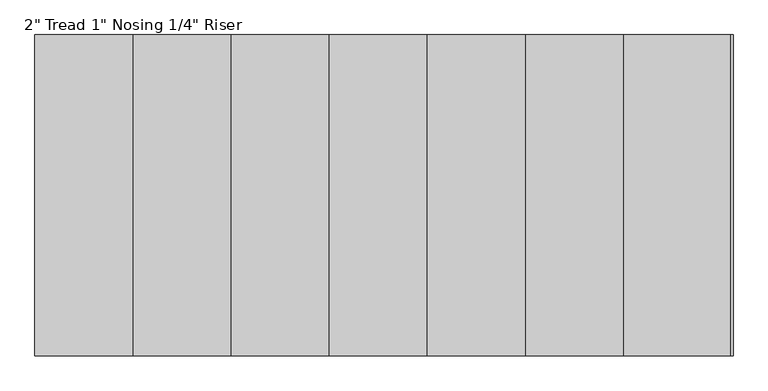
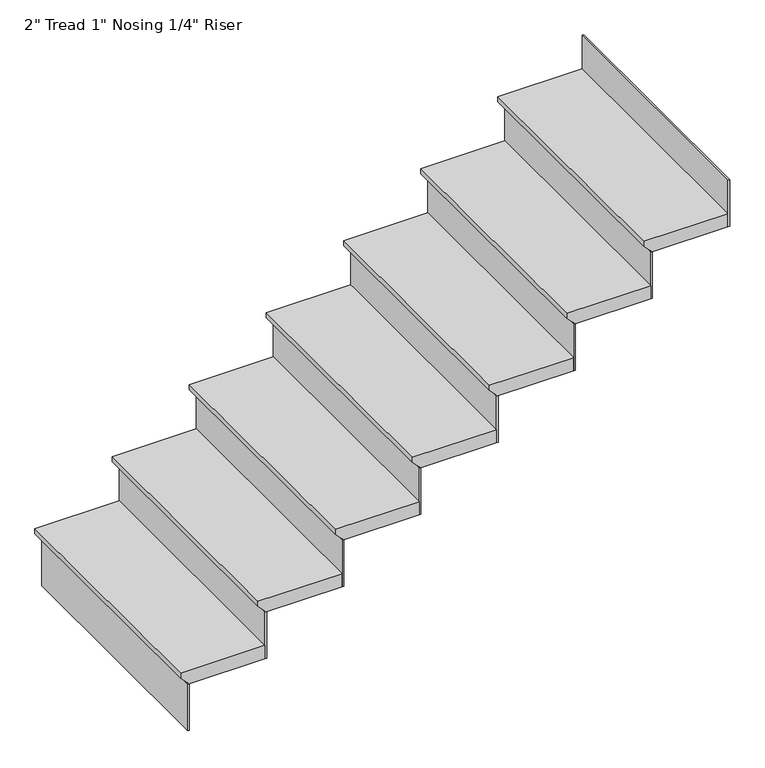
"""IFC4 building model written with IfcOpenShell, lengths in millimetres: stair flight geometry."""

from ifc_helpers import new_model, si_unit, frame, origin, place, context, project, spatial, polyline, outline, extrude, source, transform, mapped, element, save


def stair_flight_9d0467a4(model_context):
    return source(origin(), model_context, "Body", "SweptSolid", [
        extrude(outline(polyline([(8966.2, -11753.6120641), (8966.2, -12058.4120641), (8947.15, -12058.4120641), (8921.75, -12033.0120641), (8915.4, -12033.0120641), (8915.4, -11753.6120641), (8966.2, -11753.6120641)])), frame((0.0, -4817.9038196, 0.0), z_axis=(0.0, 1.0, 0.0), x_axis=(0.0, 0.0, 1.0)), (0.0, 0.0, 1.0), 914.4),
        extrude(outline(polyline([(-12026.6620641, -4817.9038196), (-12033.0120641, -4817.9038196), (-12033.0120641, -3903.5038196), (-12026.6620641, -3903.5038196), (-12026.6620641, -4817.9038196)])), frame((0.0, 0.0, 8737.6), z_axis=(0.0, 0.0, 1.0), x_axis=(1.0, 0.0, 0.0)), (0.0, 0.0, 1.0), 177.8),
        extrude(outline(polyline([(-11747.2620641, -4817.9038196), (-11753.6120641, -4817.9038196), (-11753.6120641, -3903.5038196), (-11747.2620641, -3903.5038196), (-11747.2620641, -4817.9038196)])), frame((0.0, 0.0, 8915.4), z_axis=(0.0, 0.0, 1.0), x_axis=(1.0, 0.0, 0.0)), (0.0, 0.0, 1.0), 177.8),
        extrude(outline(polyline([(9144.0, -11474.2120641), (9144.0, -11779.0120641), (9124.95, -11779.0120641), (9099.55, -11753.6120641), (9093.2, -11753.6120641), (9093.2, -11474.2120641), (9144.0, -11474.2120641)])), frame((0.0, -4817.9038196, 0.0), z_axis=(0.0, 1.0, 0.0), x_axis=(0.0, 0.0, 1.0)), (0.0, 0.0, 1.0), 914.4),
        extrude(outline(polyline([(-11467.8620641, -4817.9038196), (-11474.2120641, -4817.9038196), (-11474.2120641, -3903.5038196), (-11467.8620641, -3903.5038196), (-11467.8620641, -4817.9038196)])), frame((0.0, 0.0, 9093.2), z_axis=(0.0, 0.0, 1.0), x_axis=(1.0, 0.0, 0.0)), (0.0, 0.0, 1.0), 177.8),
        extrude(outline(polyline([(9321.8, -11194.8120641), (9321.8, -11499.6120641), (9302.75, -11499.6120641), (9277.35, -11474.2120641), (9271.0, -11474.2120641), (9271.0, -11194.8120641), (9321.8, -11194.8120641)])), frame((0.0, -4817.9038196, 0.0), z_axis=(0.0, 1.0, 0.0), x_axis=(0.0, 0.0, 1.0)), (0.0, 0.0, 1.0), 914.4),
        extrude(outline(polyline([(-11188.4620641, -4817.9038196), (-11194.8120641, -4817.9038196), (-11194.8120641, -3903.5038196), (-11188.4620641, -3903.5038196), (-11188.4620641, -4817.9038196)])), frame((0.0, 0.0, 9271.0), z_axis=(0.0, 0.0, 1.0), x_axis=(1.0, 0.0, 0.0)), (0.0, 0.0, 1.0), 177.8),
        extrude(outline(polyline([(9499.6, -10915.4120641), (9499.6, -11220.2120641), (9480.55, -11220.2120641), (9455.15, -11194.8120641), (9448.8, -11194.8120641), (9448.8, -10915.4120641), (9499.6, -10915.4120641)])), frame((0.0, -4817.9038196, 0.0), z_axis=(0.0, 1.0, 0.0), x_axis=(0.0, 0.0, 1.0)), (0.0, 0.0, 1.0), 914.4),
        extrude(outline(polyline([(-10909.0620641, -4817.9038196), (-10915.4120641, -4817.9038196), (-10915.4120641, -3903.5038196), (-10909.0620641, -3903.5038196), (-10909.0620641, -4817.9038196)])), frame((0.0, 0.0, 9448.8), z_axis=(0.0, 0.0, 1.0), x_axis=(1.0, 0.0, 0.0)), (0.0, 0.0, 1.0), 177.8),
        extrude(outline(polyline([(9677.4, -10636.0120641), (9677.4, -10940.8120641), (9658.35, -10940.8120641), (9632.95, -10915.4120641), (9626.6, -10915.4120641), (9626.6, -10636.0120641), (9677.4, -10636.0120641)])), frame((0.0, -4817.9038196, 0.0), z_axis=(0.0, 1.0, 0.0), x_axis=(0.0, 0.0, 1.0)), (0.0, 0.0, 1.0), 914.4),
        extrude(outline(polyline([(-10629.6620641, -4817.9038196), (-10636.0120641, -4817.9038196), (-10636.0120641, -3903.5038196), (-10629.6620641, -3903.5038196), (-10629.6620641, -4817.9038196)])), frame((0.0, 0.0, 9626.6), z_axis=(0.0, 0.0, 1.0), x_axis=(1.0, 0.0, 0.0)), (0.0, 0.0, 1.0), 177.8),
        extrude(outline(polyline([(9855.2, -10356.6120641), (9855.2, -10661.4120641), (9836.15, -10661.4120641), (9810.75, -10636.0120641), (9804.4, -10636.0120641), (9804.4, -10356.6120641), (9855.2, -10356.6120641)])), frame((0.0, -4817.9038196, 0.0), z_axis=(0.0, 1.0, 0.0), x_axis=(0.0, 0.0, 1.0)), (0.0, 0.0, 1.0), 914.4),
        extrude(outline(polyline([(-10350.2620641, -4817.9038196), (-10356.6120641, -4817.9038196), (-10356.6120641, -3903.5038196), (-10350.2620641, -3903.5038196), (-10350.2620641, -4817.9038196)])), frame((0.0, 0.0, 9804.4), z_axis=(0.0, 0.0, 1.0), x_axis=(1.0, 0.0, 0.0)), (0.0, 0.0, 1.0), 177.8),
        extrude(outline(polyline([(-10070.8620641, -4817.9038196), (-10077.2120641, -4817.9038196), (-10077.2120641, -3903.5038196), (-10070.8620641, -3903.5038196), (-10070.8620641, -4817.9038196)])), frame((0.0, 0.0, 9982.2), z_axis=(0.0, 0.0, 1.0), x_axis=(1.0, 0.0, 0.0)), (0.0, 0.0, 1.0), 177.8),
        extrude(outline(polyline([(10033.0, -10077.2120641), (10033.0, -10382.0120641), (10013.95, -10382.0120641), (9988.55, -10356.6120641), (9982.2, -10356.6120641), (9982.2, -10077.2120641), (10033.0, -10077.2120641)])), frame((0.0, -4817.9038196, 0.0), z_axis=(0.0, 1.0, 0.0), x_axis=(0.0, 0.0, 1.0)), (0.0, 0.0, 1.0), 914.4),
    ])


if __name__ == "__main__":
    model = new_model("IFC4")
    model_context = context("Model", 3, world=origin())
    ifc_project = project(units=[si_unit("LENGTHUNIT", "METRE", prefix="MILLI")], contexts=[model_context])
    site = spatial("IfcSite", under=ifc_project)
    building = spatial("IfcBuilding", under=site)
    placement = place(None, origin())
    stair_flight_shape = stair_flight_9d0467a4(model_context)
    element("IfcStairFlight", 1, ObjectType="2\" Tread 1\" Nosing 1/4\" Riser", at=placement, inside=building, context=model_context, shape_type="MappedRepresentation", body=[
        mapped(stair_flight_shape, transform((0.0, 0.0, 0.0), x_axis=(1.0, 0.0, 0.0), y_axis=(0.0, 1.0, 0.0), z_axis=(0.0, 0.0, 1.0))),
    ])
    save(model, "model.ifc")
